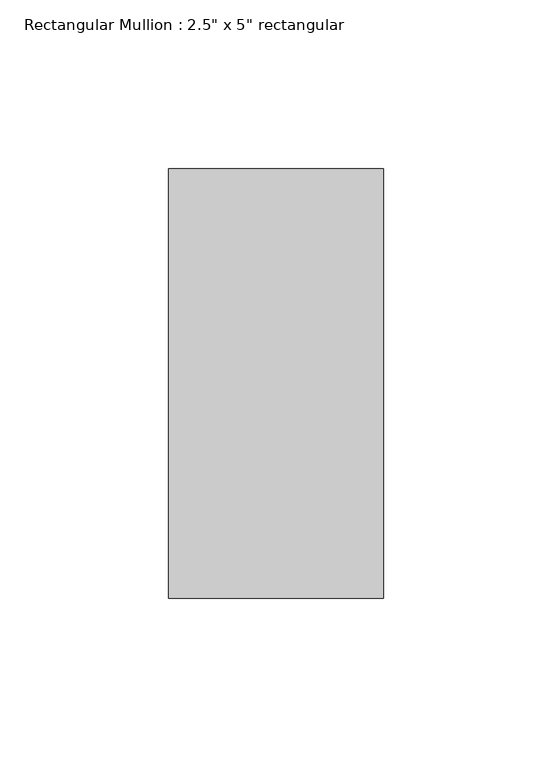
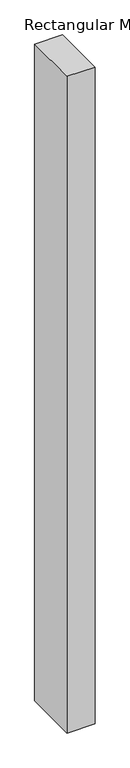
"""IFC4 building model written with IfcOpenShell, lengths in millimetres: member geometry."""

from ifc_helpers import new_model, si_unit, frame, origin, place, context, project, spatial, polyline, outline, extrude, source, transform, mapped, element, save


def member_90febb00(model_context):
    return source(origin(), model_context, "Body", "SweptSolid", [
        extrude(outline(polyline([(31.75, 63.5), (31.75, -63.5), (-31.75, -63.5), (-31.75, 63.5), (31.75, 63.5)])), frame((0.0, 0.0, -1571.3949481), z_axis=(0.0, 0.0, 1.0), x_axis=(1.0, 0.0, 0.0)), (0.0, 0.0, 1.0), 1571.3949481),
    ])


if __name__ == "__main__":
    model = new_model("IFC4")
    model_context = context("Model", 3, world=origin())
    ifc_project = project(units=[si_unit("LENGTHUNIT", "METRE", prefix="MILLI")], contexts=[model_context])
    site = spatial("IfcSite", under=ifc_project)
    building = spatial("IfcBuilding", under=site)
    placement = place(None, origin())
    member_shape = member_90febb00(model_context)
    element("IfcMember", 1, ObjectType="Rectangular Mullion : 2.5\" x 5\" rectangular", at=placement, inside=building, context=model_context, shape_type="MappedRepresentation", body=[
        mapped(member_shape, transform((0.0, 0.0, 0.0), x_axis=(1.0, 0.0, 0.0), y_axis=(0.0, 1.0, 0.0), z_axis=(0.0, 0.0, 1.0))),
    ])
    save(model, "model.ifc")

# Revit data of these elements
# Type "Rectangular Mullion : 2.5\" x 5\" rectangular"
#   built-in parameter 1007304 = 0.416667 (stored number, unit not read)
#   built-in parameter 1007301 = 0.104167 (stored number, unit not read)
#   built-in parameter 1007300 = 0.104167 (stored number, unit not read)
# Element 1 (IfcMember, "Rectangular Mullion : 2.5\" x 5\" rectangular")
#   Materials on its faces: "Aluminum"
# Materials
#   "Aluminum": class "Metal", colour RGB 247 247 247, transparency 0, Description = "Aluminum 6061", Cost = 0
